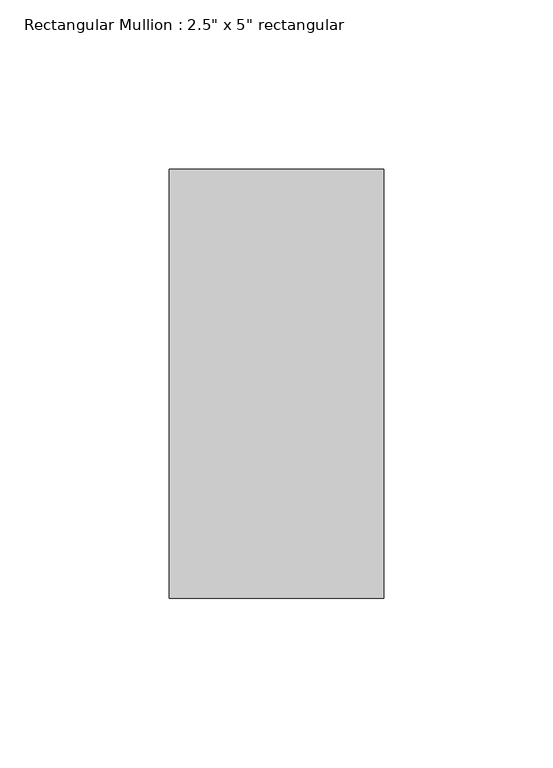
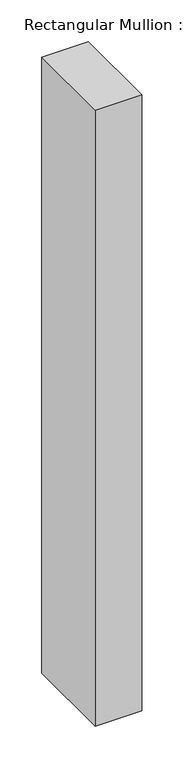
"""IFC4 building model written with IfcOpenShell, lengths in millimetres: member geometry."""

from ifc_helpers import new_model, si_unit, frame, origin, place, context, project, spatial, polyline, outline, extrude, source, transform, mapped, element, save


def member_50c8646f(model_context):
    return source(origin(), model_context, "Body", "SweptSolid", [
        extrude(outline(polyline([(31.75, 63.5), (31.75, -63.5), (-31.75, -63.5), (-31.75, 63.5), (31.75, 63.5)])), frame((0.0, 0.0, -894.9490947), z_axis=(0.0, 0.0, 1.0), x_axis=(1.0, 0.0, 0.0)), (0.0, 0.0, 1.0), 894.9490947),
    ])


if __name__ == "__main__":
    model = new_model("IFC4")
    model_context = context("Model", 3, world=origin())
    ifc_project = project(units=[si_unit("LENGTHUNIT", "METRE", prefix="MILLI")], contexts=[model_context])
    site = spatial("IfcSite", under=ifc_project)
    building = spatial("IfcBuilding", under=site)
    placement = place(None, origin())
    member_shape = member_50c8646f(model_context)
    element("IfcMember", 1, ObjectType="Rectangular Mullion : 2.5\" x 5\" rectangular", at=placement, inside=building, context=model_context, shape_type="MappedRepresentation", body=[
        mapped(member_shape, transform((0.0, 0.0, 0.0), x_axis=(1.0, 0.0, 0.0), y_axis=(0.0, 1.0, 0.0), z_axis=(0.0, 0.0, 1.0))),
    ])
    save(model, "model.ifc")

# Revit data of these elements
# Type "Rectangular Mullion : 2.5\" x 5\" rectangular"
#   built-in parameter 1007304 = 0.416667 (stored number, unit not read)
#   built-in parameter 1007301 = 0.104167 (stored number, unit not read)
#   built-in parameter 1007300 = 0.104167 (stored number, unit not read)
# Element 1 (IfcMember, "Rectangular Mullion : 2.5\" x 5\" rectangular")
#   Materials on its faces: "Aluminum"
# Materials
#   "Aluminum": class "Metal", colour RGB 247 247 247, transparency 0, Description = "Aluminum 6061", Cost = 0
